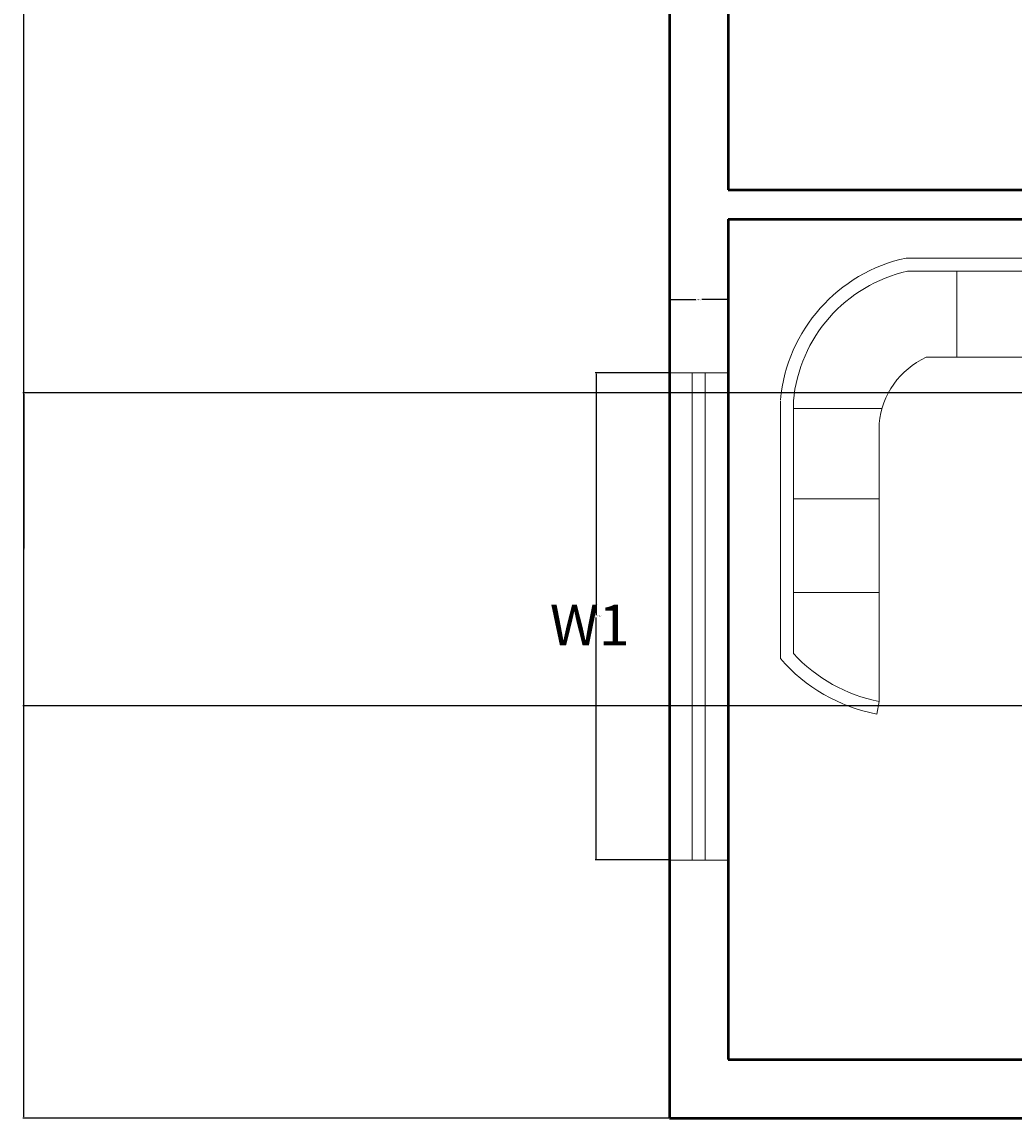
# Model space of a CAD drawing. Units: inches. Extents: x 7359 to 7979, y 33027 to 34263.
# Tile 20 of 32: x 7359 to 7511, y 33765 to 33933. Entities that reach past the tile are written whole.
import ezdxf

# ---------------------------------------------------------------- set-up
doc = ezdxf.new("R2010")
doc.units = ezdxf.units.IN
for name, color, linetype, lineweight in [('A-ANNO-DIMS', 2, 'Continuous', 18), ('A-ANNO-TEXT', 3, 'Continuous', 18), ('A-FURN', 8, 'Continuous', 18), ('A-GLAZ', 4, 'Continuous', 18), ('A-WALL', 7, 'Continuous', 50)]:
    doc.layers.add(name, color=color, linetype=linetype, lineweight=lineweight)
doc.styles.get("Standard").update_dxf_attribs({"font": 'arial.ttf'})
doc.dimstyles.get("Standard").update_dxf_attribs({"dimtxt": 0.18, "dimasz": 0.18, "dimexe": 0.18, "dimexo": 0.0625, "dimgap": 0.09, "dimtad": 0, "dimtih": 1, "dimtoh": 1, "dimdec": 4, "dimzin": 0, "dimdsep": 46, "dimtxsty": 'Standard', "dimcen": 0.09, "dimadec": 0, "dimazin": 0, "dimtfac": 1, "dimtdec": 4, "dimtofl": 0, "dimtmove": 0, "dimatfit": 3, "dimfxl": 1, "dimtolj": 1, "dimtzin": 0, "dimarcsym": 0})

# ---------------------------------------------------------------- blocks, each defined once
blk = doc.blocks.new('SOFA-CORNER')
for p, q in [((19.3, 69.98), (52.27, 69.98)), ((19.51, 67.98), (51.43, 67.98)), ((27.06, 54.75), (27.06, 67.98)), ((42.86, 54.75), (42.86, 67.98)), ((22.35, 54.75), (58.44, 54.75)), ((58.44, 54.75), (60.39, 55.17)), ((0, 8.53), (0, 48.06)), ((2, 9.3), (2, 48.06)), ((15.59, 46.88), (2, 46.88)), ((15.16, 44.58), (15.16, 1.96)), ((15.16, 33.02), (2, 33.02)), ((15.16, 18.66), (2, 18.66)), ((14.78, 0), (15.16, 1.96))]:
    blk.add_line(p, q)
for centre, radius, start, end in [((24.48, 45.95), 24.58, 102.1798, 174.6548), ((31.37, 48.88), 29.7, 12.2304, 45.2702), ((24.48, 45.95), 22.58, 102.7099, 174.6548), ((31.37, 48.88), 27.7, 12.2304, 43.5923), ((27.51, 43.47), 12.4, 114.5692, 174.8439), ((19.72, 25.63), 26.1, 220.9183, 259.0828), ((19.72, 25.63), 24.1, 222.6619, 259.0828)]:
    blk.add_arc(centre, radius, start, end)
blk = doc.blocks.new('WINDOW-W1-DRAWING-SIDE')
for p, q in [((0, 74.75), (9, 74.75)), ((3.5, 0), (3.5, 74.75)), ((5.5, 0), (5.5, 74.75)), ((0, 0), (9, 0))]:
    blk.add_line(p, q)
blk = doc.blocks.new('*D60')
at = {"layer": 'A-ANNO-DIMS', "color": 0, "lineweight": -2, "transparency": 16777216}
for p, q in [((7458.53, 33879.18), (7447.2, 33879.18)), ((7447.38, 33879), (7447.38, 33841.98)), ((7447.38, 33804.61), (7447.38, 33841.62)), ((7458.53, 33804.43), (7447.2, 33804.43))]:
    blk.add_line(p, q, dxfattribs=at)
at = {"layer": 'A-ANNO-DIMS', "color": 0, "transparency": 16777216}
for points in [[(7447.35, 33879), (7447.41, 33879), (7447.38, 33879.18)], [(7447.35, 33804.61), (7447.41, 33804.61), (7447.38, 33804.43)]]:
    blk.add_solid(points, dxfattribs=at)
at = {"layer": 'Defpoints', "color": 0, "transparency": 16777216}
for p in [(7447.38, 33879.18), (7458.59, 33879.18), (7458.59, 33804.43)]:
    blk.add_point(p, dxfattribs=at)
at = {"layer": 'A-ANNO-DIMS', "color": 0, "transparency": 16777216, "insert": (7447.38, 33841.8), "char_height": 0.18, "attachment_point": 5}
blk.add_mtext('\\A1;SIDE W1 75 TYP.', dxfattribs=at)
blk = doc.blocks.new('*D61')
at = {"layer": 'A-ANNO-DIMS', "color": 0, "lineweight": -2, "transparency": 16777216}
for p, q in [((7458.59, 33879.24), (7458.59, 33890.57)), ((7458.77, 33890.39), (7462.63, 33890.39)), ((7467.41, 33890.39), (7463.55, 33890.39)), ((7467.59, 33879.24), (7467.59, 33890.57))]:
    blk.add_line(p, q, dxfattribs=at)
at = {"layer": 'A-ANNO-DIMS', "color": 0, "transparency": 16777216}
for points in [[(7458.77, 33890.42), (7458.77, 33890.36), (7458.59, 33890.39)], [(7467.41, 33890.42), (7467.41, 33890.36), (7467.59, 33890.39)]]:
    blk.add_solid(points, dxfattribs=at)
at = {"layer": 'Defpoints', "color": 0, "transparency": 16777216}
for p in [(7467.59, 33890.39), (7458.59, 33879.18), (7467.59, 33879.18)]:
    blk.add_point(p, dxfattribs=at)
at = {"layer": 'A-ANNO-DIMS', "color": 0, "transparency": 16777216, "insert": (7463.09, 33890.39), "char_height": 0.18, "attachment_point": 5}
blk.add_mtext('\\A1;9 TYP.', dxfattribs=at)
blk = doc.blocks.new('*D65')
at = {"layer": 'A-ANNO-DIMS', "color": 0, "lineweight": -2, "transparency": 16777216}
for p, q in [((7458.53, 34233.33), (7359.41, 34233.33)), ((7359.59, 34233.15), (7359.59, 33999.27)), ((7359.59, 33765.01), (7359.59, 33998.9)), ((7458.53, 33764.83), (7359.41, 33764.83))]:
    blk.add_line(p, q, dxfattribs=at)
at = {"layer": 'A-ANNO-DIMS', "color": 0, "transparency": 16777216}
for points in [[(7359.56, 34233.15), (7359.62, 34233.15), (7359.59, 34233.33)], [(7359.56, 33765.01), (7359.62, 33765.01), (7359.59, 33764.83)]]:
    blk.add_solid(points, dxfattribs=at)
at = {"layer": 'Defpoints', "color": 0, "transparency": 16777216}
for p in [(7359.59, 34233.33), (7458.59, 34233.33), (7458.59, 33764.83)]:
    blk.add_point(p, dxfattribs=at)
at = {"layer": 'A-ANNO-DIMS', "color": 0, "transparency": 16777216, "insert": (7359.59, 33999.08), "char_height": 0.18, "attachment_point": 5}
blk.add_mtext('\\A1;468.5', dxfattribs=at)
blk = doc.blocks.new('*D72')
at = {"layer": 'A-ANNO-DIMS', "color": 0, "lineweight": -2, "transparency": 16777216}
for p, q in [((7689.43, 33876.08), (7359.41, 33876.08)), ((7359.59, 33875.9), (7359.59, 33852.27)), ((7359.59, 33828.26), (7359.59, 33851.9)), ((7689.43, 33828.08), (7359.41, 33828.08))]:
    blk.add_line(p, q, dxfattribs=at)
at = {"layer": 'A-ANNO-DIMS', "color": 0, "transparency": 16777216}
for points in [[(7359.56, 33875.9), (7359.62, 33875.9), (7359.59, 33876.08)], [(7359.56, 33828.26), (7359.62, 33828.26), (7359.59, 33828.08)]]:
    blk.add_solid(points, dxfattribs=at)
at = {"layer": 'Defpoints', "color": 0, "transparency": 16777216}
for p in [(7359.59, 33876.08), (7689.49, 33876.08), (7689.49, 33828.08)]:
    blk.add_point(p, dxfattribs=at)
at = {"layer": 'A-ANNO-DIMS', "color": 0, "transparency": 16777216, "insert": (7359.59, 33852.08), "char_height": 0.18, "attachment_point": 5}
blk.add_mtext('\\A1;48', dxfattribs=at)

msp = doc.modelspace()

# ---------------------------------------------------------------- linework, layer by layer
at = {"layer": 'A-WALL'}
for p, q in [((7458.5915, 34233.3339), (7458.5915, 33764.8339)), ((7467.5915, 34077.3339), (7467.5915, 33907.2339)), ((7467.5915, 33907.2339), (7641.4915, 33907.2339)), ((7467.5915, 33902.7339), (7641.4915, 33902.7339)), ((7467.5915, 33902.7339), (7467.5915, 33773.8339)), ((7467.5915, 33773.8339), (7689.4915, 33773.8339)), ((7458.5915, 33764.8339), (7883.9915, 33764.8339))]:
    msp.add_line(p, q, dxfattribs=at)

# ---------------------------------------------------------------- block references
at = {"layer": 'A-FURN'}
msp.add_blockref('SOFA-CORNER', (7475.615, 33826.797), dxfattribs=at)
at = {"layer": 'A-GLAZ'}
msp.add_blockref('WINDOW-W1-DRAWING-SIDE', (7458.591, 33804.425), dxfattribs=at)

# ---------------------------------------------------------------- texts
at = {"layer": 'A-ANNO-TEXT'}
msp.add_text('W1', height=6.25941, dxfattribs=at).set_placement((7440.2572, 33837.3361))

# ---------------------------------------------------------------- dimensions: what is measured, and where the dimension line sits
at = {"layer": 'A-ANNO-DIMS'}
for base, p1, p2, override, picture, middle in [((7359.5866, 34233.3339), (7458.5915, 33764.8339), (7458.5915, 34233.3339), {"dimdec": 1, "dimlfac": 1, "dimrnd": 0, "dimzin": 0, "dimdsep": 46, "dimlunit": 2}, '*D65', (7359.5866, 33999.0839)), ((7359.5866, 33876.0839), (7689.4915, 33828.0839), (7689.4915, 33876.0839), {"dimdec": 0, "dimlfac": 1, "dimrnd": 0, "dimzin": 0, "dimdsep": 46, "dimlunit": 2}, '*D72', (7359.5866, 33852.0839))]:
    dim = msp.add_linear_dim(base=base, p1=p1, p2=p2, angle=90, dimstyle='Standard', override=override, dxfattribs=at)
    dim.commit()
    dim.dimension.update_dxf_attribs({"geometry": picture, "text_midpoint": middle})
dim = msp.add_linear_dim(base=(7467.5915, 33890.3891), p1=(7458.5915, 33879.1764), p2=(7467.5915, 33879.1764), text='<> TYP.', dimstyle='Standard', override={"dimdec": 0, "dimlfac": 1, "dimrnd": 0, "dimzin": 0, "dimdsep": 46, "dimlunit": 2}, dxfattribs=at)
dim.commit()
dim.dimension.update_dxf_attribs({"geometry": '*D61', "text_midpoint": (7463.0915, 33890.3891)})
dim = msp.add_linear_dim(base=(7447.3788, 33879.1764), p1=(7458.5915, 33804.4254), p2=(7458.5915, 33879.1764), angle=90, text='SIDE W1 <> TYP.', dimstyle='Standard', override={"dimdec": 0, "dimlfac": 1, "dimrnd": 0, "dimzin": 0, "dimdsep": 46, "dimlunit": 2}, dxfattribs=at)
dim.commit()
dim.dimension.update_dxf_attribs({"geometry": '*D60', "text_midpoint": (7447.3788, 33841.8009)})

doc.saveas('drawing.dxf')
